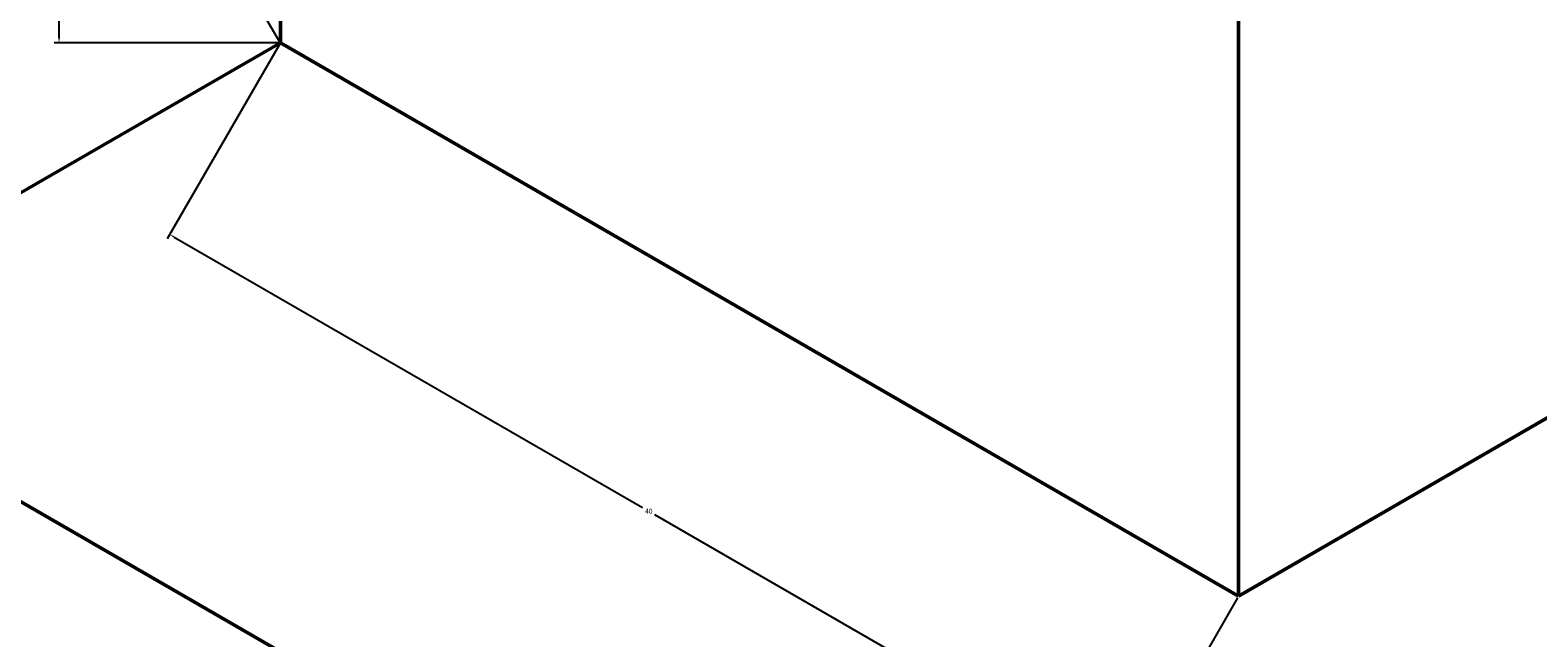
# Model space of a CAD drawing. Units: millimetres. Extents: x 2919 to 3075, y 2801 to 2951.
# Tile 4 of 14: x 2952 to 3006, y 2854 to 2876. Entities that reach past the tile are written whole.
import ezdxf

# ---------------------------------------------------------------- set-up
doc = ezdxf.new("R2010")
doc.units = ezdxf.units.MM
doc.layers.add('M-DIMS', color=2, linetype='Continuous', lineweight=18)
doc.layers.add('M-OUTL', color=7, linetype='Continuous', lineweight=50)
doc.styles.get("Standard").update_dxf_attribs({"font": 'arial.ttf'})
doc.dimstyles.get("Standard").update_dxf_attribs({"dimtxt": 0.18, "dimasz": 0.18, "dimexe": 0.18, "dimexo": 0.0625, "dimgap": 0.09, "dimtad": 0, "dimtih": 1, "dimtoh": 1, "dimdec": 4, "dimzin": 0, "dimdsep": 46, "dimtxsty": 'Standard', "dimcen": 0.09, "dimadec": 0, "dimazin": 0, "dimtfac": 1, "dimtdec": 4, "dimtofl": 0, "dimtmove": 0, "dimatfit": 3, "dimfxl": 1, "dimtolj": 1, "dimtzin": 0, "dimarcsym": 0})

# ---------------------------------------------------------------- blocks, each defined once
blk = doc.blocks.new('*D1')
at = {"layer": 'Defpoints', "color": 0, "transparency": 16777216}
for p in [(2987.323, 2944.203), (3074.337, 2944.203), (3010.912, 2808.893)]:
    blk.add_point(p, dxfattribs=at)
at = {"layer": 'M-DIMS', "color": 0, "lineweight": -2, "transparency": 16777216}
for p, q in [((2987.386, 2944.203), (3074.517, 2944.203)), ((3074.337, 2944.023), (3074.337, 2876.73)), ((3074.337, 2809.073), (3074.337, 2876.366)), ((3010.974, 2808.893), (3074.517, 2808.893))]:
    blk.add_line(p, q, dxfattribs=at)
at = {"layer": 'M-DIMS', "color": 0, "transparency": 16777216}
for points in [[(3074.307, 2944.023), (3074.367, 2944.023), (3074.337, 2944.203)], [(3074.307, 2809.073), (3074.367, 2809.073), (3074.337, 2808.893)]]:
    blk.add_solid(points, dxfattribs=at)
at = {"layer": 'M-DIMS', "color": 0, "transparency": 16777216, "insert": (3074.337, 2876.548), "char_height": 0.18, "attachment_point": 5}
blk.add_mtext('\\A1;135.3', dxfattribs=at)
blk = doc.blocks.new('*D2')
at = {"layer": 'Defpoints', "color": 0, "transparency": 16777216}
for p in [(2927.773, 2856.893), (3066.337, 2840.893), (3066.337, 2800.893)]:
    blk.add_point(p, dxfattribs=at)
at = {"layer": 'M-DIMS', "color": 0, "lineweight": -2, "transparency": 16777216}
for p, q in [((2927.773, 2856.831), (2927.773, 2800.713)), ((3066.337, 2840.831), (3066.337, 2800.713)), ((2927.953, 2800.893), (2996.6, 2800.893)), ((3066.157, 2800.893), (2997.51, 2800.893))]:
    blk.add_line(p, q, dxfattribs=at)
at = {"layer": 'M-DIMS', "color": 0, "transparency": 16777216}
for points in [[(2927.953, 2800.923), (2927.953, 2800.863), (2927.773, 2800.893)], [(3066.157, 2800.923), (3066.157, 2800.863), (3066.337, 2800.893)]]:
    blk.add_solid(points, dxfattribs=at)
at = {"layer": 'M-DIMS', "color": 0, "transparency": 16777216, "insert": (2997.055, 2800.893), "char_height": 0.18, "attachment_point": 5}
blk.add_mtext('\\A1;138.56', dxfattribs=at)
blk = doc.blocks.new('*D3')
at = {"layer": 'Defpoints', "color": 0, "transparency": 16777216}
for p in [(2927.773, 2856.893), (2923.773, 2849.965), (3010.912, 2808.893)]:
    blk.add_point(p, dxfattribs=at)
at = {"layer": 'M-DIMS', "color": 0, "lineweight": -2, "transparency": 16777216}
for p, q in [((2927.742, 2856.839), (2923.683, 2849.809)), ((2923.929, 2849.875), (2965.124, 2826.091)), ((3006.756, 2802.055), (2965.561, 2825.839)), ((3010.88, 2808.839), (3006.822, 2801.809))]:
    blk.add_line(p, q, dxfattribs=at)
at = {"layer": 'M-DIMS', "color": 0, "transparency": 16777216}
for points in [[(2923.944, 2849.901), (2923.914, 2849.849), (2923.773, 2849.965)], [(3006.771, 2802.081), (3006.741, 2802.029), (3006.912, 2801.965)]]:
    blk.add_solid(points, dxfattribs=at)
at = {"layer": 'M-DIMS', "color": 0, "transparency": 16777216, "insert": (2965.342, 2825.965), "char_height": 0.18, "attachment_point": 5}
blk.add_mtext('\\A1;96', dxfattribs=at)
blk = doc.blocks.new('*D10')
at = {"layer": 'Defpoints', "color": 0, "transparency": 16777216}
for p in [(2956.682, 2882.821), (2960.682, 2875.893), (2941.63, 2864.893)]:
    blk.add_point(p, dxfattribs=at)
at = {"layer": 'M-DIMS', "color": 0, "lineweight": -2, "transparency": 16777216}
for p, q in [((2956.526, 2882.731), (2947.375, 2877.448)), ((2960.651, 2875.947), (2956.592, 2882.977)), ((2937.785, 2871.911), (2946.936, 2877.195)), ((2941.598, 2864.947), (2937.54, 2871.977))]:
    blk.add_line(p, q, dxfattribs=at)
at = {"layer": 'M-DIMS', "color": 0, "transparency": 16777216}
for points in [[(2956.511, 2882.757), (2956.541, 2882.705), (2956.682, 2882.821)], [(2937.77, 2871.937), (2937.8, 2871.885), (2937.63, 2871.821)]]:
    blk.add_solid(points, dxfattribs=at)
at = {"layer": 'M-DIMS', "color": 0, "transparency": 16777216, "insert": (2947.156, 2877.321), "char_height": 0.18, "attachment_point": 5}
blk.add_mtext('\\A1;22', dxfattribs=at)
blk = doc.blocks.new('*D11')
at = {"layer": 'Defpoints', "color": 0, "transparency": 16777216}
for p in [(2960.682, 2875.893), (2956.682, 2868.965), (2995.323, 2855.893)]:
    blk.add_point(p, dxfattribs=at)
at = {"layer": 'M-DIMS', "color": 0, "lineweight": -2, "transparency": 16777216}
for p, q in [((2960.651, 2875.839), (2956.592, 2868.809)), ((2956.838, 2868.875), (2973.78, 2859.093)), ((2991.167, 2849.055), (2974.225, 2858.837)), ((2995.292, 2855.839), (2991.233, 2848.809))]:
    blk.add_line(p, q, dxfattribs=at)
at = {"layer": 'M-DIMS', "color": 0, "transparency": 16777216}
for points in [[(2956.853, 2868.901), (2956.823, 2868.849), (2956.682, 2868.965)], [(2991.182, 2849.081), (2991.152, 2849.029), (2991.323, 2848.965)]]:
    blk.add_solid(points, dxfattribs=at)
at = {"layer": 'M-DIMS', "color": 0, "transparency": 16777216, "insert": (2974.003, 2858.965), "char_height": 0.18, "attachment_point": 5}
blk.add_mtext('\\A1;40', dxfattribs=at)
blk = doc.blocks.new('*D13')
at = {"layer": 'Defpoints', "color": 0, "transparency": 16777216}
for p in [(2952.682, 2903.893), (2960.682, 2903.893), (2960.682, 2875.893)]:
    blk.add_point(p, dxfattribs=at)
at = {"layer": 'M-DIMS', "color": 0, "lineweight": -2, "transparency": 16777216}
for p, q in [((2960.62, 2903.893), (2952.502, 2903.893)), ((2952.682, 2903.713), (2952.682, 2890.075)), ((2952.682, 2876.073), (2952.682, 2889.711)), ((2960.62, 2875.893), (2952.502, 2875.893))]:
    blk.add_line(p, q, dxfattribs=at)
at = {"layer": 'M-DIMS', "color": 0, "transparency": 16777216}
for points in [[(2952.652, 2903.713), (2952.712, 2903.713), (2952.682, 2903.893)], [(2952.652, 2876.073), (2952.712, 2876.073), (2952.682, 2875.893)]]:
    blk.add_solid(points, dxfattribs=at)
at = {"layer": 'M-DIMS', "color": 0, "transparency": 16777216, "insert": (2952.682, 2889.893), "char_height": 0.18, "attachment_point": 5}
blk.add_mtext('\\A1;28', dxfattribs=at)

msp = doc.modelspace()

# ---------------------------------------------------------------- linework, layer by layer
at = {"layer": 'M-OUTL'}
for p, q in [((2960.6821, 2875.8932), (2960.6821, 2903.8932)), ((2995.3232, 2855.8932), (2995.3232, 2883.8932)), ((2941.6296, 2864.8932), (2960.6821, 2875.8932)), ((2941.6296, 2864.8932), (2960.6821, 2875.8932)), ((2941.6296, 2864.8932), (2960.6821, 2875.8932)), ((2960.6821, 2875.8932), (2995.3232, 2855.8932)), ((2995.3232, 2855.8932), (3021.3039, 2870.8932)), ((3010.9116, 2824.8932), (2941.6296, 2864.8932))]:
    msp.add_line(p, q, dxfattribs=at)

# ---------------------------------------------------------------- dimensions: what is measured, and where the dimension line sits
at = {"layer": 'M-DIMS'}
for base, p1, p2, angle, override, picture, middle in [((3074.3372, 2944.2026), (3010.9116, 2808.8932), (2987.3232, 2944.2026), 90, {"dimdec": 1, "dimlfac": 1, "dimrnd": 0, "dimzin": 0, "dimdsep": 46, "dimlunit": 2}, '*D1', (3074.3372, 2876.5479)), ((2952.6821, 2903.8932), (2960.6821, 2875.8932), (2960.6821, 2903.8932), 90, {"dimdec": 0, "dimlfac": 1, "dimrnd": 0, "dimzin": 0, "dimdsep": 46, "dimlunit": 2}, '*D13', (2952.6821, 2889.8932)), ((2956.6821, 2882.8214), (2941.6296, 2864.8932), (2960.6821, 2875.8932), 30, {"dimdec": 0, "dimlfac": 1, "dimrnd": 0, "dimzin": 0, "dimdsep": 46, "dimlunit": 2}, '*D10', (2947.1559, 2877.3214)), ((2956.6821, 2868.965), (2995.3232, 2855.8932), (2960.6821, 2875.8932), 150, {"dimdec": 0, "dimlfac": 1, "dimrnd": 0, "dimzin": 0, "dimdsep": 46, "dimlunit": 2}, '*D11', (2974.0027, 2858.965)), ((2923.7732, 2849.965), (3010.9116, 2808.8932), (2927.7732, 2856.8932), 150, {"dimdec": 0, "dimlfac": 1, "dimrnd": 0, "dimzin": 0, "dimdsep": 46, "dimlunit": 2}, '*D3', (2965.3424, 2825.965))]:
    dim = msp.add_linear_dim(base=base, p1=p1, p2=p2, angle=angle, dimstyle='Standard', override=override, dxfattribs=at)
    dim.commit()
    dim.dimension.update_dxf_attribs({"geometry": picture, "text_midpoint": middle})
dim = msp.add_linear_dim(base=(3066.3372, 2800.8932), p1=(2927.7732, 2856.8932), p2=(3066.3372, 2840.8932), dimstyle='Standard', override={"dimdec": 2, "dimlfac": 1, "dimrnd": 0, "dimzin": 0, "dimdsep": 46, "dimlunit": 2}, dxfattribs=at)
dim.commit()
dim.dimension.update_dxf_attribs({"geometry": '*D2', "text_midpoint": (2997.0552, 2800.8932)})

doc.saveas('drawing.dxf')
